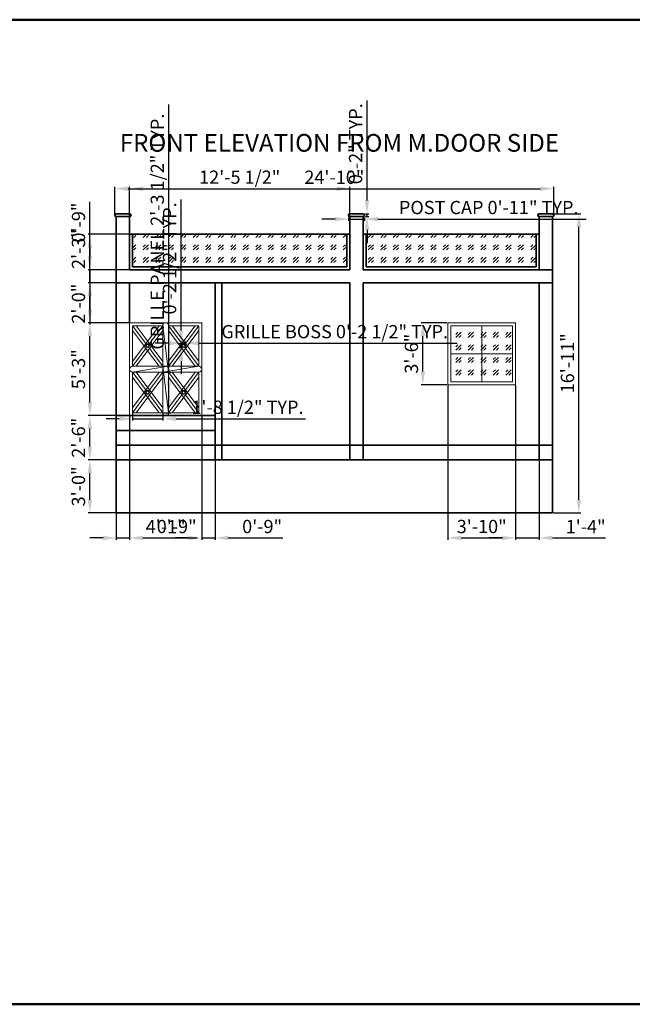
# Model space of a CAD drawing. Units: inches. Extents: x 2113 to 4530, y 1685 to 2353.
# Tile 5 of 6: x 2836 to 3252, y 1685 to 2353. Entities that reach past the tile are written whole.
import ezdxf

# ---------------------------------------------------------------- set-up
doc = ezdxf.new("R2010")
doc.units = ezdxf.units.IN
for name, color, linetype, lineweight in [('A-ANNO-TITL', 7, 'Continuous', 35), ('A-ANNO-TTLB', 7, 'Continuous', 50), ('A-ELEV', 7, 'Continuous', 35), ('A-ELEV-DOOR', 3, 'Continuous', 18), ('A-ELEV-GLAZ', 4, 'Continuous', 18), ('A-ELEV-PATT', 9, 'Continuous', 13), ('S-ANNO-DIMS', 2, 'Continuous', 18)]:
    doc.layers.add(name, color=color, linetype=linetype, lineweight=lineweight)
doc.styles.get("Standard").update_dxf_attribs({"font": 'arial.ttf'})
doc.dimstyles.new('ISO-25', dxfattribs={"dimtxt": 9, "dimasz": 9, "dimexe": 1.25, "dimexo": 0.625, "dimgap": 2, "dimtad": 1, "dimdec": 1, "dimlunit": 4, "dimtxsty": 'Standard', "dimcen": 2.5, "dimazin": 0, "dimtfac": 1, "dimtdec": 1, "dimtmove": 0, "dimatfit": 3, "dimfxl": 1, "dimarcsym": 0})

# ---------------------------------------------------------------- blocks, each defined once
blk = doc.blocks.new('PARAPET-POST-CAP')
for p, q in [((1, 2), (10, 2)), ((1, 0), (10, 0))]:
    blk.add_line(p, q)
for centre, start, end in [((1, 1), 90, 270), ((10, 1), 270, 90)]:
    blk.add_arc(centre, 1, start, end)
blk = doc.blocks.new('ENTRY-GRILLE-X')
for p, q in [((0, 27.5), (9, 15.42)), ((0, 3.35), (18.01, 27.5)), ((2.49, 27.5), (20.5, 3.35)), ((11.5, 15.42), (20.5, 27.5)), ((0, 24.15), (18.01, 0)), ((2.49, 0), (20.5, 24.15)), ((0, 0), (9, 12.08)), ((11.5, 12.08), (20.5, 0))]:
    blk.add_line(p, q)
blk = doc.blocks.new('ENTRY-GRILLE-BOSS')
for centre, radius in [((1.35, 1.34), 1.34), ((1.35, 1.39), 0.848)]:
    blk.add_circle(centre, radius)
blk = doc.blocks.new('*D44')
at = {"layer": 'Defpoints', "color": 0, "transparency": 16777216}
for p in [(2946.26, 2133.15), (2948.95, 2133.55), (2948.95, 2133.15)]:
    blk.add_point(p, dxfattribs=at)
at = {"layer": 'S-ANNO-DIMS', "color": 0, "lineweight": -2, "transparency": 16777216}
for p, q in [((2937.26, 2133.55), (2928.26, 2133.55)), ((2946.26, 2133.78), (2946.26, 2134.8)), ((2946.26, 2133.55), (2948.95, 2133.55)), ((2948.95, 2133.78), (2948.95, 2134.8)), ((2957.95, 2133.55), (3133.28, 2133.55))]:
    blk.add_line(p, q, dxfattribs=at)
at = {"layer": 'S-ANNO-DIMS', "color": 0, "transparency": 16777216}
for points in [[(2937.26, 2135.05), (2937.26, 2132.05), (2946.26, 2133.55)], [(2957.95, 2135.05), (2957.95, 2132.05), (2948.95, 2133.55)]]:
    blk.add_solid(points, dxfattribs=at)
at = {"layer": 'S-ANNO-DIMS', "color": 0, "transparency": 16777216, "insert": (3050.12, 2140.21), "char_height": 9, "attachment_point": 5}
blk.add_mtext('GRILLE BOSS 0\'-2 1/2" TYP.', dxfattribs=at)
blk = doc.blocks.new('*D45')
at = {"layer": 'Defpoints', "color": 0, "transparency": 16777216}
for p in [(2945.86, 2133.15), (2946.26, 2133.15), (2946.26, 2130.46)]:
    blk.add_point(p, dxfattribs=at)
at = {"layer": 'S-ANNO-DIMS', "color": 0, "lineweight": -2, "transparency": 16777216}
for p, q in [((2945.86, 2142.15), (2945.86, 2230.98)), ((2945.64, 2133.15), (2944.61, 2133.15)), ((2945.64, 2130.46), (2944.61, 2130.46)), ((2945.86, 2130.46), (2945.86, 2133.15)), ((2945.86, 2121.46), (2945.86, 2112.46))]:
    blk.add_line(p, q, dxfattribs=at)
at = {"layer": 'S-ANNO-DIMS', "color": 0, "transparency": 16777216}
for points in [[(2944.36, 2142.15), (2947.36, 2142.15), (2945.86, 2133.15)], [(2944.36, 2121.46), (2947.36, 2121.46), (2945.86, 2130.46)]]:
    blk.add_solid(points, dxfattribs=at)
at = {"layer": 'S-ANNO-DIMS', "color": 0, "transparency": 16777216, "insert": (2939.21, 2191.07), "char_height": 9, "attachment_point": 5, "rotation": 90}
blk.add_mtext('0\'-2 1/2" TYP.', dxfattribs=at)
blk = doc.blocks.new('*D46')
at = {"layer": 'Defpoints', "color": 0, "transparency": 16777216}
for p in [(3059.4, 2219.4), (3070.4, 2219.4), (3070.4, 2217.75)]:
    blk.add_point(p, dxfattribs=at)
at = {"layer": 'S-ANNO-DIMS', "color": 0, "lineweight": -2, "transparency": 16777216}
for p, q in [((3050.4, 2217.75), (3041.4, 2217.75)), ((3059.4, 2218.77), (3059.4, 2216.5)), ((3059.4, 2217.75), (3070.4, 2217.75)), ((3070.4, 2218.77), (3070.4, 2216.5)), ((3079.4, 2217.75), (3220.88, 2217.75))]:
    blk.add_line(p, q, dxfattribs=at)
at = {"layer": 'S-ANNO-DIMS', "color": 0, "transparency": 16777216}
for points in [[(3050.4, 2219.25), (3050.4, 2216.25), (3059.4, 2217.75)], [(3079.4, 2219.25), (3079.4, 2216.25), (3070.4, 2217.75)]]:
    blk.add_solid(points, dxfattribs=at)
at = {"layer": 'S-ANNO-DIMS', "color": 0, "transparency": 16777216, "insert": (3154.64, 2224.4), "char_height": 9, "attachment_point": 5}
blk.add_mtext('POST CAP 0\'-11" TYP.', dxfattribs=at)
blk = doc.blocks.new('*D47')
at = {"layer": 'Defpoints', "color": 0, "transparency": 16777216}
for p in [(3070.4, 2221.4), (3070.4, 2219.4), (3072.05, 2221.4)]:
    blk.add_point(p, dxfattribs=at)
at = {"layer": 'S-ANNO-DIMS', "color": 0, "lineweight": -2, "transparency": 16777216}
for p, q in [((3072.05, 2230.4), (3072.05, 2298.26)), ((3071.03, 2221.4), (3073.3, 2221.4)), ((3071.03, 2219.4), (3073.3, 2219.4)), ((3072.05, 2219.4), (3072.05, 2221.4)), ((3072.05, 2210.4), (3072.05, 2201.4))]:
    blk.add_line(p, q, dxfattribs=at)
at = {"layer": 'S-ANNO-DIMS', "color": 0, "transparency": 16777216}
for points in [[(3070.55, 2230.4), (3073.55, 2230.4), (3072.05, 2221.4)], [(3070.55, 2210.4), (3073.55, 2210.4), (3072.05, 2219.4)]]:
    blk.add_solid(points, dxfattribs=at)
at = {"layer": 'S-ANNO-DIMS', "color": 0, "transparency": 16777216, "insert": (3065.46, 2268.83), "char_height": 9, "attachment_point": 5, "rotation": 90}
blk.add_mtext('0\'-2" TYP.', dxfattribs=at)
blk = doc.blocks.new('*D48')
at = {"layer": 'Defpoints', "color": 0, "transparency": 16777216}
for p in [(2933.4, 2113.9), (2937.53, 2113.9), (2933.4, 2086.4)]:
    blk.add_point(p, dxfattribs=at)
at = {"layer": 'S-ANNO-DIMS', "color": 0, "lineweight": -2, "transparency": 16777216}
for p, q in [((2937.53, 2113.9), (2937.53, 2295.52)), ((2934.03, 2113.9), (2938.78, 2113.9)), ((2937.53, 2095.4), (2937.53, 2104.9)), ((2934.03, 2086.4), (2938.78, 2086.4))]:
    blk.add_line(p, q, dxfattribs=at)
at = {"layer": 'S-ANNO-DIMS', "color": 0, "transparency": 16777216}
for points in [[(2936.03, 2104.9), (2939.03, 2104.9), (2937.53, 2113.9)], [(2936.03, 2095.4), (2939.03, 2095.4), (2937.53, 2086.4)]]:
    blk.add_solid(points, dxfattribs=at)
at = {"layer": 'S-ANNO-DIMS', "color": 0, "transparency": 16777216, "insert": (2930.87, 2209.21), "char_height": 9, "attachment_point": 5, "rotation": 90}
blk.add_mtext('GRILLE PANEL 2\'-3 1/2" TYP.', dxfattribs=at)
blk = doc.blocks.new('*D49')
at = {"layer": 'Defpoints', "color": 0, "transparency": 16777216}
for p in [(2912.9, 2086.4), (2933.4, 2086.4), (2933.4, 2082.27)]:
    blk.add_point(p, dxfattribs=at)
at = {"layer": 'S-ANNO-DIMS', "color": 0, "lineweight": -2, "transparency": 16777216}
for p, q in [((2912.9, 2085.77), (2912.9, 2081.02)), ((2933.4, 2085.77), (2933.4, 2081.02)), ((2903.9, 2082.27), (2894.9, 2082.27)), ((2912.9, 2082.27), (2933.4, 2082.27)), ((2942.4, 2082.27), (3030.39, 2082.27))]:
    blk.add_line(p, q, dxfattribs=at)
at = {"layer": 'S-ANNO-DIMS', "color": 0, "transparency": 16777216}
for points in [[(2903.9, 2083.77), (2903.9, 2080.77), (2912.9, 2082.27)], [(2942.4, 2083.77), (2942.4, 2080.77), (2933.4, 2082.27)]]:
    blk.add_solid(points, dxfattribs=at)
at = {"layer": 'S-ANNO-DIMS', "color": 0, "transparency": 16777216, "insert": (2990.89, 2088.92), "char_height": 9, "attachment_point": 5}
blk.add_mtext('1\'-8 1/2" TYP.', dxfattribs=at)
blk = doc.blocks.new('*D64')
at = {"layer": 'Defpoints', "color": 0, "transparency": 16777216}
for p in [(2883.95, 2054.4), (2901.9, 2054.4), (2901.9, 2018.4)]:
    blk.add_point(p, dxfattribs=at)
at = {"layer": 'S-ANNO-DIMS', "color": 0, "lineweight": -2, "transparency": 16777216}
for p, q in [((2901.28, 2054.4), (2882.7, 2054.4)), ((2883.95, 2027.4), (2883.95, 2045.4)), ((2901.28, 2018.4), (2882.7, 2018.4))]:
    blk.add_line(p, q, dxfattribs=at)
at = {"layer": 'S-ANNO-DIMS', "color": 0, "transparency": 16777216}
for points in [[(2882.45, 2045.4), (2885.45, 2045.4), (2883.95, 2054.4)], [(2882.45, 2027.4), (2885.45, 2027.4), (2883.95, 2018.4)]]:
    blk.add_solid(points, dxfattribs=at)
at = {"layer": 'S-ANNO-DIMS', "color": 0, "transparency": 16777216, "insert": (2877.35, 2036.4), "char_height": 9, "attachment_point": 5, "rotation": 90}
blk.add_mtext('3\'-0"', dxfattribs=at)
blk = doc.blocks.new('*D65')
at = {"layer": 'Defpoints', "color": 0, "transparency": 16777216}
for p in [(2883.95, 2084.4), (2901.9, 2084.4), (2901.9, 2054.4)]:
    blk.add_point(p, dxfattribs=at)
at = {"layer": 'S-ANNO-DIMS', "color": 0, "lineweight": -2, "transparency": 16777216}
for p, q in [((2901.28, 2084.4), (2882.7, 2084.4)), ((2883.95, 2063.4), (2883.95, 2075.4)), ((2901.28, 2054.4), (2882.7, 2054.4))]:
    blk.add_line(p, q, dxfattribs=at)
at = {"layer": 'S-ANNO-DIMS', "color": 0, "transparency": 16777216}
for points in [[(2882.45, 2075.4), (2885.45, 2075.4), (2883.95, 2084.4)], [(2882.45, 2063.4), (2885.45, 2063.4), (2883.95, 2054.4)]]:
    blk.add_solid(points, dxfattribs=at)
at = {"layer": 'S-ANNO-DIMS', "color": 0, "transparency": 16777216, "insert": (2877.36, 2069.4), "char_height": 9, "attachment_point": 5, "rotation": 90}
blk.add_mtext('2\'-6"', dxfattribs=at)
blk = doc.blocks.new('*D66')
at = {"layer": 'Defpoints', "color": 0, "transparency": 16777216}
for p in [(2883.95, 2147.4), (2910.9, 2147.4), (2910.9, 2084.4)]:
    blk.add_point(p, dxfattribs=at)
at = {"layer": 'S-ANNO-DIMS', "color": 0, "lineweight": -2, "transparency": 16777216}
for p, q in [((2910.28, 2147.4), (2882.7, 2147.4)), ((2883.95, 2093.4), (2883.95, 2138.4)), ((2910.28, 2084.4), (2882.7, 2084.4))]:
    blk.add_line(p, q, dxfattribs=at)
at = {"layer": 'S-ANNO-DIMS', "color": 0, "transparency": 16777216}
for points in [[(2882.45, 2138.4), (2885.45, 2138.4), (2883.95, 2147.4)], [(2882.45, 2093.4), (2885.45, 2093.4), (2883.95, 2084.4)]]:
    blk.add_solid(points, dxfattribs=at)
at = {"layer": 'S-ANNO-DIMS', "color": 0, "transparency": 16777216, "insert": (2877.35, 2115.9), "char_height": 9, "attachment_point": 5, "rotation": 90}
blk.add_mtext('5\'-3"', dxfattribs=at)
blk = doc.blocks.new('*D67')
at = {"layer": 'Defpoints', "color": 0, "transparency": 16777216}
for p in [(2883.95, 2174.4), (2910.9, 2174.4), (2910.9, 2147.4)]:
    blk.add_point(p, dxfattribs=at)
at = {"layer": 'S-ANNO-DIMS', "color": 0, "lineweight": -2, "transparency": 16777216}
for p, q in [((2883.95, 2174.4), (2883.95, 2211.47)), ((2910.28, 2174.4), (2882.7, 2174.4)), ((2883.95, 2156.4), (2883.95, 2165.4)), ((2910.28, 2147.4), (2882.7, 2147.4))]:
    blk.add_line(p, q, dxfattribs=at)
at = {"layer": 'S-ANNO-DIMS', "color": 0, "transparency": 16777216}
for points in [[(2882.45, 2165.4), (2885.45, 2165.4), (2883.95, 2174.4)], [(2882.45, 2156.4), (2885.45, 2156.4), (2883.95, 2147.4)]]:
    blk.add_solid(points, dxfattribs=at)
at = {"layer": 'S-ANNO-DIMS', "color": 0, "transparency": 16777216, "insert": (2877.35, 2197.44), "char_height": 9, "attachment_point": 5, "rotation": 90}
blk.add_mtext('2\'-3"', dxfattribs=at)
blk = doc.blocks.new('*D68')
at = {"layer": 'Defpoints', "color": 0, "transparency": 16777216}
for p in [(2883.95, 2183.4), (2910.9, 2183.4), (2910.9, 2174.4)]:
    blk.add_point(p, dxfattribs=at)
at = {"layer": 'S-ANNO-DIMS', "color": 0, "lineweight": -2, "transparency": 16777216}
for p, q in [((2883.95, 2192.4), (2883.95, 2229.32)), ((2910.28, 2183.4), (2882.7, 2183.4)), ((2883.95, 2174.4), (2883.95, 2183.4)), ((2910.28, 2174.4), (2882.7, 2174.4)), ((2883.95, 2165.4), (2883.95, 2156.4))]:
    blk.add_line(p, q, dxfattribs=at)
at = {"layer": 'S-ANNO-DIMS', "color": 0, "transparency": 16777216}
for points in [[(2882.45, 2192.4), (2885.45, 2192.4), (2883.95, 2183.4)], [(2882.45, 2165.4), (2885.45, 2165.4), (2883.95, 2174.4)]]:
    blk.add_solid(points, dxfattribs=at)
at = {"layer": 'S-ANNO-DIMS', "color": 0, "transparency": 16777216, "insert": (2877.36, 2215.36), "char_height": 9, "attachment_point": 5, "rotation": 90}
blk.add_mtext('0\'-9"', dxfattribs=at)
blk = doc.blocks.new('*D69')
at = {"layer": 'Defpoints', "color": 0, "transparency": 16777216}
for p in [(2910.9, 2084.4), (2959.9, 2084.4), (2959.9, 2001.45)]:
    blk.add_point(p, dxfattribs=at)
at = {"layer": 'S-ANNO-DIMS', "color": 0, "lineweight": -2, "transparency": 16777216}
for p, q in [((2910.9, 2083.77), (2910.9, 2000.2)), ((2959.9, 2083.77), (2959.9, 2000.2)), ((2919.9, 2001.45), (2950.9, 2001.45))]:
    blk.add_line(p, q, dxfattribs=at)
at = {"layer": 'S-ANNO-DIMS', "color": 0, "transparency": 16777216}
for points in [[(2919.9, 2002.95), (2919.9, 1999.95), (2910.9, 2001.45)], [(2950.9, 2002.95), (2950.9, 1999.95), (2959.9, 2001.45)]]:
    blk.add_solid(points, dxfattribs=at)
at = {"layer": 'S-ANNO-DIMS', "color": 0, "transparency": 16777216, "insert": (2935.4, 2007.96), "char_height": 9, "attachment_point": 5}
blk.add_mtext('4\'-1"', dxfattribs=at)
blk = doc.blocks.new('*D70')
at = {"layer": 'Defpoints', "color": 0, "transparency": 16777216}
for p in [(2901.9, 2084.4), (2910.9, 2084.4), (2910.9, 2001.45)]:
    blk.add_point(p, dxfattribs=at)
at = {"layer": 'S-ANNO-DIMS', "color": 0, "lineweight": -2, "transparency": 16777216}
for p, q in [((2901.9, 2083.77), (2901.9, 2000.2)), ((2910.9, 2083.77), (2910.9, 2000.2)), ((2892.9, 2001.45), (2883.9, 2001.45)), ((2901.9, 2001.45), (2910.9, 2001.45)), ((2919.9, 2001.45), (2956.83, 2001.45))]:
    blk.add_line(p, q, dxfattribs=at)
at = {"layer": 'S-ANNO-DIMS', "color": 0, "transparency": 16777216}
for points in [[(2892.9, 2002.95), (2892.9, 1999.95), (2901.9, 2001.45)], [(2919.9, 2002.95), (2919.9, 1999.95), (2910.9, 2001.45)]]:
    blk.add_solid(points, dxfattribs=at)
at = {"layer": 'S-ANNO-DIMS', "color": 0, "transparency": 16777216, "insert": (2942.86, 2008.04), "char_height": 9, "attachment_point": 5}
blk.add_mtext('0\'-9"', dxfattribs=at)
blk = doc.blocks.new('*D71')
at = {"layer": 'Defpoints', "color": 0, "transparency": 16777216}
for p in [(2959.9, 2084.4), (2968.9, 2084.4), (2968.9, 2001.45)]:
    blk.add_point(p, dxfattribs=at)
at = {"layer": 'S-ANNO-DIMS', "color": 0, "lineweight": -2, "transparency": 16777216}
for p, q in [((2959.9, 2083.77), (2959.9, 2000.2)), ((2968.9, 2083.77), (2968.9, 2000.2)), ((2950.9, 2001.45), (2941.9, 2001.45)), ((2959.9, 2001.45), (2968.9, 2001.45)), ((2977.9, 2001.45), (3014.83, 2001.45))]:
    blk.add_line(p, q, dxfattribs=at)
at = {"layer": 'S-ANNO-DIMS', "color": 0, "transparency": 16777216}
for points in [[(2950.9, 2002.95), (2950.9, 1999.95), (2959.9, 2001.45)], [(2977.9, 2002.95), (2977.9, 1999.95), (2968.9, 2001.45)]]:
    blk.add_solid(points, dxfattribs=at)
at = {"layer": 'S-ANNO-DIMS', "color": 0, "transparency": 16777216, "insert": (3000.86, 2008.04), "char_height": 9, "attachment_point": 5}
blk.add_mtext('0\'-9"', dxfattribs=at)
blk = doc.blocks.new('*D72')
at = {"layer": 'Defpoints', "color": 0, "transparency": 16777216}
for p in [(3126.9, 2105.4), (3172.9, 2105.4), (3172.9, 2001.45)]:
    blk.add_point(p, dxfattribs=at)
at = {"layer": 'S-ANNO-DIMS', "color": 0, "lineweight": -2, "transparency": 16777216}
for p, q in [((3126.9, 2104.77), (3126.9, 2000.2)), ((3172.9, 2104.77), (3172.9, 2000.2)), ((3135.9, 2001.45), (3163.9, 2001.45))]:
    blk.add_line(p, q, dxfattribs=at)
at = {"layer": 'S-ANNO-DIMS', "color": 0, "transparency": 16777216}
for points in [[(3135.9, 2002.95), (3135.9, 1999.95), (3126.9, 2001.45)], [(3163.9, 2002.95), (3163.9, 1999.95), (3172.9, 2001.45)]]:
    blk.add_solid(points, dxfattribs=at)
at = {"layer": 'S-ANNO-DIMS', "color": 0, "transparency": 16777216, "insert": (3149.9, 2008.04), "char_height": 9, "attachment_point": 5}
blk.add_mtext('3\'-10"', dxfattribs=at)
blk = doc.blocks.new('*D73')
at = {"layer": 'Defpoints', "color": 0, "transparency": 16777216}
for p in [(3109.95, 2147.4), (3126.9, 2147.4), (3126.9, 2105.4)]:
    blk.add_point(p, dxfattribs=at)
at = {"layer": 'S-ANNO-DIMS', "color": 0, "lineweight": -2, "transparency": 16777216}
for p, q in [((3126.28, 2147.4), (3108.7, 2147.4)), ((3109.95, 2114.4), (3109.95, 2138.4)), ((3126.28, 2105.4), (3108.7, 2105.4))]:
    blk.add_line(p, q, dxfattribs=at)
at = {"layer": 'S-ANNO-DIMS', "color": 0, "transparency": 16777216}
for points in [[(3108.45, 2138.4), (3111.45, 2138.4), (3109.95, 2147.4)], [(3108.45, 2114.4), (3111.45, 2114.4), (3109.95, 2105.4)]]:
    blk.add_solid(points, dxfattribs=at)
at = {"layer": 'S-ANNO-DIMS', "color": 0, "transparency": 16777216, "insert": (3103.35, 2126.4), "char_height": 9, "attachment_point": 5, "rotation": 90}
blk.add_mtext('3\'-6"', dxfattribs=at)
blk = doc.blocks.new('*D74')
at = {"layer": 'Defpoints', "color": 0, "transparency": 16777216}
for p in [(3172.9, 2105.4), (3188.9, 2054.4), (3188.9, 2001.45)]:
    blk.add_point(p, dxfattribs=at)
at = {"layer": 'S-ANNO-DIMS', "color": 0, "lineweight": -2, "transparency": 16777216}
for p, q in [((3172.9, 2104.77), (3172.9, 2000.2)), ((3188.9, 2053.77), (3188.9, 2000.2)), ((3163.9, 2001.45), (3154.9, 2001.45)), ((3172.9, 2001.45), (3188.9, 2001.45)), ((3197.9, 2001.45), (3233.98, 2001.45))]:
    blk.add_line(p, q, dxfattribs=at)
at = {"layer": 'S-ANNO-DIMS', "color": 0, "transparency": 16777216}
for points in [[(3163.9, 2002.95), (3163.9, 1999.95), (3172.9, 2001.45)], [(3197.9, 2002.95), (3197.9, 1999.95), (3188.9, 2001.45)]]:
    blk.add_solid(points, dxfattribs=at)
at = {"layer": 'S-ANNO-DIMS', "color": 0, "transparency": 16777216, "insert": (3220.44, 2007.96), "char_height": 9, "attachment_point": 5}
blk.add_mtext('1\'-4"', dxfattribs=at)
blk = doc.blocks.new('*D75')
at = {"layer": 'Defpoints', "color": 0, "transparency": 16777216}
for p in [(3060.4, 2238.35), (2910.9, 2183.4), (3060.4, 2183.4)]:
    blk.add_point(p, dxfattribs=at)
at = {"layer": 'S-ANNO-DIMS', "color": 0, "lineweight": -2, "transparency": 16777216}
for p, q in [((2910.9, 2184.02), (2910.9, 2239.6)), ((2919.9, 2238.35), (3051.4, 2238.35)), ((3060.4, 2184.02), (3060.4, 2239.6))]:
    blk.add_line(p, q, dxfattribs=at)
at = {"layer": 'S-ANNO-DIMS', "color": 0, "transparency": 16777216}
for points in [[(2919.9, 2239.85), (2919.9, 2236.85), (2910.9, 2238.35)], [(3051.4, 2239.85), (3051.4, 2236.85), (3060.4, 2238.35)]]:
    blk.add_solid(points, dxfattribs=at)
at = {"layer": 'S-ANNO-DIMS', "color": 0, "transparency": 16777216, "insert": (2985.65, 2245), "char_height": 9, "attachment_point": 5}
blk.add_mtext('12\'-5 1/2"', dxfattribs=at)
blk = doc.blocks.new('*D76')
at = {"layer": 'Defpoints', "color": 0, "transparency": 16777216}
for p in [(2910.9, 2207.4), (2883.95, 2183.4), (2910.9, 2183.4)]:
    blk.add_point(p, dxfattribs=at)
at = {"layer": 'S-ANNO-DIMS', "color": 0, "lineweight": -2, "transparency": 16777216}
for p, q in [((2910.28, 2207.4), (2882.7, 2207.4)), ((2883.95, 2198.4), (2883.95, 2192.4)), ((2910.28, 2183.4), (2882.7, 2183.4)), ((2883.95, 2183.4), (2883.95, 2146.32))]:
    blk.add_line(p, q, dxfattribs=at)
at = {"layer": 'S-ANNO-DIMS', "color": 0, "transparency": 16777216}
for points in [[(2882.45, 2198.4), (2885.45, 2198.4), (2883.95, 2207.4)], [(2882.45, 2192.4), (2885.45, 2192.4), (2883.95, 2183.4)]]:
    blk.add_solid(points, dxfattribs=at)
at = {"layer": 'S-ANNO-DIMS', "color": 0, "transparency": 16777216, "insert": (2877.36, 2160.36), "char_height": 9, "attachment_point": 5, "rotation": 90}
blk.add_mtext('2\'-0"', dxfattribs=at)
blk = doc.blocks.new('*D77')
at = {"layer": 'Defpoints', "color": 0, "transparency": 16777216}
for p in [(3198.9, 2238.35), (2900.9, 2220.4), (3198.9, 2220.4)]:
    blk.add_point(p, dxfattribs=at)
at = {"layer": 'S-ANNO-DIMS', "color": 0, "lineweight": -2, "transparency": 16777216}
for p, q in [((2900.9, 2221.02), (2900.9, 2239.6)), ((2909.9, 2238.35), (3189.9, 2238.35)), ((3198.9, 2221.02), (3198.9, 2239.6))]:
    blk.add_line(p, q, dxfattribs=at)
at = {"layer": 'S-ANNO-DIMS', "color": 0, "transparency": 16777216}
for points in [[(2909.9, 2239.85), (2909.9, 2236.85), (2900.9, 2238.35)], [(3189.9, 2239.85), (3189.9, 2236.85), (3198.9, 2238.35)]]:
    blk.add_solid(points, dxfattribs=at)
at = {"layer": 'S-ANNO-DIMS', "color": 0, "transparency": 16777216, "insert": (3049.9, 2244.94), "char_height": 9, "attachment_point": 5}
blk.add_mtext('24\'-10"', dxfattribs=at)
blk = doc.blocks.new('*D78')
at = {"layer": 'Defpoints', "color": 0, "transparency": 16777216}
for p in [(3197.9, 2221.4), (3215.85, 2221.4), (3197.9, 2018.4)]:
    blk.add_point(p, dxfattribs=at)
at = {"layer": 'S-ANNO-DIMS', "color": 0, "lineweight": -2, "transparency": 16777216}
for p, q in [((3198.53, 2221.4), (3217.1, 2221.4)), ((3215.85, 2027.4), (3215.85, 2212.4)), ((3198.53, 2018.4), (3217.1, 2018.4))]:
    blk.add_line(p, q, dxfattribs=at)
at = {"layer": 'S-ANNO-DIMS', "color": 0, "transparency": 16777216}
for points in [[(3214.35, 2212.4), (3217.35, 2212.4), (3215.85, 2221.4)], [(3214.35, 2027.4), (3217.35, 2027.4), (3215.85, 2018.4)]]:
    blk.add_solid(points, dxfattribs=at)
at = {"layer": 'S-ANNO-DIMS', "color": 0, "transparency": 16777216, "insert": (3209.26, 2119.9), "char_height": 9, "attachment_point": 5, "rotation": 90}
blk.add_mtext('16\'-11"', dxfattribs=at)

msp = doc.modelspace()

# ---------------------------------------------------------------- hatches: boundary and pattern name
at = {"layer": 'A-ELEV-PATT'}
h = msp.add_hatch(dxfattribs=at)
h.set_pattern_fill('GOST_GLASS', color=256)
h.set_pattern_definition([(45, (552.7885, 677.9075), (8.485281, 0), [5, -7]), (45, (554.91, 677.9075), (8.485281, 0), [2, -10]), (45, (552.7885, 680.029), (8.485281, 0), [2, -10])])
h.paths.add_polyline_path([(3058.4, 2207.4), (2912.9, 2207.4), (2912.9, 2185.4), (3058.4, 2185.4)])
h.paths.add_polyline_path([(3186.9, 2207.4), (3071.4, 2207.4), (3071.4, 2185.4), (3186.9, 2185.4)])
h.paths.add_polyline_path([(3149.9, 2145.4), (3128.9, 2145.4), (3128.9, 2126.4), (3149.93, 2126.4)])
h.paths.add_polyline_path([(3170.9, 2145.4), (3149.9, 2145.4), (3149.93, 2126.4), (3170.9, 2126.4)])
h.paths.add_polyline_path([(3149.93, 2126.4), (3128.9, 2126.4), (3128.9, 2107.4), (3149.96, 2107.4)])
h.paths.add_polyline_path([(3170.9, 2126.4), (3149.93, 2126.4), (3149.96, 2107.4), (3170.9, 2107.4)])

# ---------------------------------------------------------------- linework, layer by layer
at = {"layer": 'A-ANNO-TTLB'}
msp.add_lwpolyline([(2112.77, 2352.97), (4498.42, 2352.97), (4498.42, 1685.12), (2112.77, 1685.12)], close=True, dxfattribs=at)
at = {"layer": 'A-ELEV'}
for p, q in [((2901.9, 2219.4), (2901.9, 2018.4)), ((2910.9, 2219.4), (2910.9, 2183.4)), ((3060.4, 2219.4), (3060.4, 2183.4)), ((3069.4, 2219.4), (3069.4, 2183.4)), ((3188.9, 2219.4), (3188.9, 2183.4)), ((3197.9, 2219.4), (3197.9, 2018.4)), ((2912.9, 2207.4), (2910.9, 2207.4)), ((2912.9, 2207.4), (2912.9, 2185.4)), ((2912.9, 2207.4), (3058.4, 2207.4)), ((3058.4, 2207.4), (3060.4, 2207.4)), ((3058.4, 2207.4), (3058.4, 2185.4)), ((3069.4, 2207.4), (3188.9, 2207.4)), ((3071.4, 2207.4), (3071.4, 2185.4)), ((3186.9, 2207.4), (3186.9, 2185.4)), ((2912.9, 2185.4), (3058.4, 2185.4)), ((3071.4, 2185.4), (3186.9, 2185.4)), ((2910.9, 2183.4), (3060.4, 2183.4)), ((3069.4, 2183.4), (3197.9, 2183.4)), ((2901.9, 2174.4), (3060.4, 2174.4)), ((2910.9, 2174.4), (2910.9, 2147.4)), ((2968.9, 2174.4), (2968.9, 2054.4)), ((2973.4, 2174.4), (2973.4, 2054.4)), ((3060.4, 2174.4), (3060.4, 2054.4)), ((3069.4, 2174.4), (3197.9, 2174.4)), ((3069.4, 2174.4), (3069.4, 2054.4)), ((3188.9, 2174.4), (3188.9, 2054.4)), ((2901.9, 2084.4), (2968.9, 2084.4)), ((2901.9, 2074.4), (2968.9, 2074.4)), ((2901.9, 2064.4), (3197.9, 2064.4)), ((2901.9, 2054.4), (3064.9, 2054.4)), ((3064.9, 2054.4), (3197.9, 2054.4)), ((2901.9, 2018.4), (3197.9, 2018.4))]:
    msp.add_line(p, q, dxfattribs=at)
at = {"layer": 'A-ELEV-DOOR'}
for p, q in [((2910.9, 2147.4), (2959.9, 2147.4)), ((2910.9, 2147.4), (2910.9, 2084.4)), ((2912.9, 2145.4), (2933.4, 2145.4)), ((2912.9, 2145.4), (2912.9, 2117.9)), ((2930.91, 2145.4), (2912.9, 2121.24)), ((2912.9, 2145.4), (2921.91, 2133.32)), ((2915.4, 2145.4), (2925.65, 2131.65)), ((2924.4, 2133.32), (2933.4, 2145.4)), ((2933.4, 2145.4), (2933.4, 2086.4)), ((2933.4, 2145.4), (2937.4, 2113.9)), ((2937.4, 2145.4), (2937.4, 2086.4)), ((2937.4, 2145.4), (2957.9, 2145.4)), ((2957.9, 2145.4), (2957.9, 2117.9)), ((2959.9, 2147.4), (2959.9, 2084.4)), ((2912.9, 2142.05), (2920.3, 2132.12)), ((2933.4, 2142.05), (2915.4, 2117.9)), ((2920.3, 2132.12), (2920.66, 2131.65)), ((2920.66, 2131.65), (2923.15, 2128.3)), ((2925.65, 2131.65), (2933.4, 2121.24)), ((2912.9, 2117.9), (2921.91, 2129.97)), ((2923.15, 2128.3), (2930.91, 2117.9)), ((2924.4, 2129.97), (2933.4, 2117.9)), ((2957.9, 2117.9), (2912.9, 2117.9)), ((2912.9, 2113.9), (2937.4, 2117.9)), ((2933.4, 2113.9), (2957.9, 2117.9)), ((2933.4, 2117.9), (2937.4, 2086.4)), ((2957.9, 2113.9), (2912.9, 2113.9)), ((2912.9, 2113.9), (2912.9, 2086.4)), ((2957.9, 2113.9), (2957.9, 2086.4)), ((2912.9, 2086.4), (2933.4, 2086.4)), ((2937.4, 2086.4), (2957.9, 2086.4))]:
    msp.add_line(p, q, dxfattribs=at)
for centre, start, end in [((2935.4, 2145.41), 0, 180), ((2912.9, 2115.9), 90, 270), ((2957.9, 2115.9), 270, 90), ((2935.4, 2086.4), 180, 0)]:
    msp.add_arc(centre, 2, start, end, dxfattribs=at)
at = {"layer": 'A-ELEV-GLAZ'}
for p, q in [((3126.9, 2147.4), (3126.9, 2105.4)), ((3126.9, 2147.4), (3172.9, 2147.4)), ((3128.9, 2145.4), (3128.9, 2107.4)), ((3128.9, 2145.4), (3170.9, 2145.4)), ((3149.9, 2145.4), (3149.96, 2107.4)), ((3170.9, 2145.4), (3170.9, 2107.4)), ((3172.9, 2147.4), (3172.9, 2105.4)), ((3128.9, 2126.4), (3170.9, 2126.4)), ((3126.9, 2105.4), (3172.9, 2105.4)), ((3128.9, 2107.4), (3170.9, 2107.4))]:
    msp.add_line(p, q, dxfattribs=at)

# ---------------------------------------------------------------- block references
at = {"layer": 'A-ELEV'}
for p in [(2900.9, 2219.4), (3059.4, 2219.4), (3187.9, 2219.4)]:
    msp.add_blockref('PARAPET-POST-CAP', p, dxfattribs=at)
at = {"layer": 'A-ELEV-DOOR'}
for name, p in [('ENTRY-GRILLE-X', (2937.4, 2117.9)), ('ENTRY-GRILLE-BOSS', (2921.7, 2130.46)), ('ENTRY-GRILLE-BOSS', (2946.26, 2130.46)), ('ENTRY-GRILLE-X', (2912.9, 2086.4)), ('ENTRY-GRILLE-X', (2937.4, 2086.4)), ('ENTRY-GRILLE-BOSS', (2921.7, 2098.82)), ('ENTRY-GRILLE-BOSS', (2946.28, 2098.82))]:
    msp.add_blockref(name, p, dxfattribs=at)

# ---------------------------------------------------------------- texts
at = {"layer": 'A-ANNO-TITL'}
msp.add_text(' FRONT ELEVATION FROM M.DOOR SIDE', height=12, dxfattribs=at).set_placement((2900.57, 2263.44))

# ---------------------------------------------------------------- dimensions: what is measured, and where the dimension line sits
at = {"layer": 'S-ANNO-DIMS'}
for base, p1, p2, text, picture, middle in [((3072.05, 2221.4), (3070.4, 2219.4), (3070.4, 2221.4), '<> TYP.', '*D47', (3065.46, 2268.83)), ((2937.53, 2113.9), (2933.4, 2086.4), (2933.4, 2113.9), 'GRILLE PANEL <> TYP.', '*D48', (2930.87, 2209.21)), ((2945.86, 2133.15), (2946.26, 2130.46), (2946.26, 2133.15), '<> TYP.', '*D45', (2939.21, 2191.07))]:
    dim = msp.add_linear_dim(base=base, p1=p1, p2=p2, angle=90, text=text, dimstyle='ISO-25', override={"dimdec": 1, "dimlfac": 1, "dimrnd": 0, "dimzin": 1, "dimdsep": 46, "dimlunit": 4, "dimfrac": 2}, dxfattribs=at)
    dim.commit()
    dim.dimension.update_dxf_attribs({"geometry": picture, "text_midpoint": middle})
for base, p1, p2, picture, middle in [((3060.4, 2238.35), (2910.9, 2183.4), (3060.4, 2183.4), '*D75', (2985.65, 2245)), ((3198.9, 2238.35), (2900.9, 2220.4), (3198.9, 2220.4), '*D77', (3049.9, 2244.94)), ((3172.9, 2001.45), (3126.9, 2105.4), (3172.9, 2105.4), '*D72', (3149.9, 2008.04)), ((3188.9, 2001.45), (3172.9, 2105.4), (3188.9, 2054.4), '*D74', (3220.44, 2007.96)), ((2910.9, 2001.45), (2901.9, 2084.4), (2910.9, 2084.4), '*D70', (2942.86, 2008.04)), ((2959.9, 2001.45), (2910.9, 2084.4), (2959.9, 2084.4), '*D69', (2935.4, 2007.96)), ((2968.9, 2001.45), (2959.9, 2084.4), (2968.9, 2084.4), '*D71', (3000.86, 2008.04))]:
    dim = msp.add_linear_dim(base=base, p1=p1, p2=p2, dimstyle='ISO-25', override={"dimdec": 1, "dimlfac": 1, "dimrnd": 0, "dimzin": 1, "dimdsep": 46, "dimlunit": 4, "dimfrac": 2}, dxfattribs=at)
    dim.commit()
    dim.dimension.update_dxf_attribs({"geometry": picture, "text_midpoint": middle})
for base, p1, p2, text, picture, middle in [((3070.4, 2217.75), (3059.4, 2219.4), (3070.4, 2219.4), 'POST CAP <> TYP.', '*D46', (3154.64, 2224.4)), ((2948.95, 2133.55), (2946.26, 2133.15), (2948.95, 2133.15), 'GRILLE BOSS <> TYP.', '*D44', (3050.12, 2140.21)), ((2933.4, 2082.27), (2912.9, 2086.4), (2933.4, 2086.4), '<> TYP.', '*D49', (2990.89, 2088.92))]:
    dim = msp.add_linear_dim(base=base, p1=p1, p2=p2, text=text, dimstyle='ISO-25', override={"dimdec": 1, "dimlfac": 1, "dimrnd": 0, "dimzin": 1, "dimdsep": 46, "dimlunit": 4, "dimfrac": 2}, dxfattribs=at)
    dim.commit()
    dim.dimension.update_dxf_attribs({"geometry": picture, "text_midpoint": middle})
for base, p1, p2, picture, middle in [((2883.95, 2183.4), (2910.9, 2174.4), (2910.9, 2183.4), '*D68', (2877.36, 2215.36)), ((3215.85, 2221.4), (3197.9, 2018.4), (3197.9, 2221.4), '*D78', (3209.26, 2119.9)), ((2883.95, 2174.4), (2910.9, 2147.4), (2910.9, 2174.4), '*D67', (2877.35, 2197.44)), ((2883.95, 2183.4), (2910.9, 2207.4), (2910.9, 2183.4), '*D76', (2877.36, 2160.36)), ((2883.95, 2147.4), (2910.9, 2084.4), (2910.9, 2147.4), '*D66', (2877.35, 2115.9)), ((3109.95, 2147.4), (3126.9, 2105.4), (3126.9, 2147.4), '*D73', (3103.35, 2126.4)), ((2883.95, 2084.4), (2901.9, 2054.4), (2901.9, 2084.4), '*D65', (2877.36, 2069.4)), ((2883.95, 2054.4), (2901.9, 2018.4), (2901.9, 2054.4), '*D64', (2877.35, 2036.4))]:
    dim = msp.add_linear_dim(base=base, p1=p1, p2=p2, angle=90, dimstyle='ISO-25', override={"dimdec": 1, "dimlfac": 1, "dimrnd": 0, "dimzin": 1, "dimdsep": 46, "dimlunit": 4, "dimfrac": 2}, dxfattribs=at)
    dim.commit()
    dim.dimension.update_dxf_attribs({"geometry": picture, "text_midpoint": middle})

doc.saveas('drawing.dxf')
